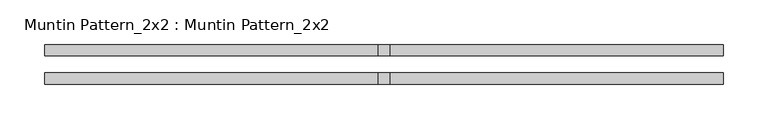
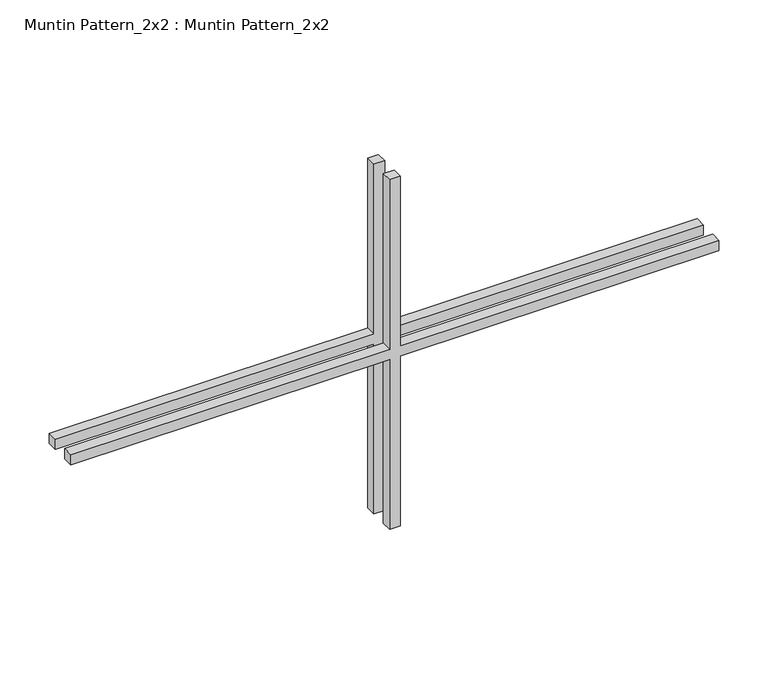
"""IFC4 building model written with IfcOpenShell, lengths in millimetres: proxy geometry, Muntin Pattern_2x2 : Muntin Pattern_2x2."""

from ifc_helpers import new_model, si_unit, frame, origin, place, context, project, spatial, polyline, outline, extrude, source, transform, mapped, element, save


def muntin_pattern_2x2_muntin_pattern_2x2_0e62f131(model_context):
    return source(origin(), model_context, "Body", "SweptSolid", [
        extrude(outline(polyline([(223.8375, -6.35), (223.8375, -381.0), (211.1375, -381.0), (211.1375, -6.35), (0.0, -6.35), (0.0, 6.35), (211.1375, 6.35), (211.1375, 381.0), (223.8375, 381.0), (223.8375, 6.35), (434.975, 6.35), (434.975, -6.35), (223.8375, -6.35)])), frame((0.0, 9.525, 0.0), z_axis=(0.0, 1.0, 0.0), x_axis=(0.0, 0.0, 1.0)), (0.0, 0.0, 1.0), 12.7),
        extrude(outline(polyline([(223.8375, -6.35), (223.8375, -381.0), (211.1375, -381.0), (211.1375, -6.35), (0.0, -6.35), (0.0, 6.35), (211.1375, 6.35), (211.1375, 381.0), (223.8375, 381.0), (223.8375, 6.35), (434.975, 6.35), (434.975, -6.35), (223.8375, -6.35)])), frame((0.0, -22.225, 0.0), z_axis=(0.0, 1.0, 0.0), x_axis=(0.0, 0.0, 1.0)), (0.0, 0.0, 1.0), 12.7),
    ])


if __name__ == "__main__":
    model = new_model("IFC4")
    model_context = context("Model", 3, world=origin())
    ifc_project = project(units=[si_unit("LENGTHUNIT", "METRE", prefix="MILLI")], contexts=[model_context])
    site = spatial("IfcSite", under=ifc_project)
    building = spatial("IfcBuilding", under=site)
    placement = place(None, origin())
    muntin_pattern_2x2_muntin_pattern_2x2_shape = muntin_pattern_2x2_muntin_pattern_2x2_0e62f131(model_context)
    element("IfcBuildingElementProxy", 1, Name="Muntin Pattern_2x2 : Muntin Pattern_2x2", ObjectType="Muntin Pattern_2x2 : Muntin Pattern_2x2", at=placement, inside=building, context=model_context, shape_type="MappedRepresentation", body=[
        mapped(muntin_pattern_2x2_muntin_pattern_2x2_shape, transform((0.0, 0.0, 0.0), x_axis=(1.0, 0.0, 0.0), y_axis=(0.0, 1.0, 0.0), z_axis=(0.0, 0.0, 1.0))),
    ])
    save(model, "model.ifc")

# Revit data of these elements
# Type "Muntin Pattern_2x2 : Muntin Pattern_2x2"
#   Width [instance default] = 4' - 0"
#   Thickness = 0' - 0 1/2"
#   Height [instance default] = 4' - 0"
#   Distance = 0' - 0 3/4"
#   Interior Material [instance default] = none
#   Exterior Material [instance default] = none
#   Default Elevation = 0
# Element 1 (IfcBuildingElementProxy, "Muntin Pattern_2x2 : Muntin Pattern_2x2")
#   Width = 2' - 6"
#   Height = 1' - 5 1/8"
#   Interior Material = Wood - Stained
#   Exterior Material = Clad - White
#   Materials on its faces: "Clad - White", "Wood - Stained"
# Materials
#   "Clad - White": class "Wood", colour RGB 242 242 238, transparency 0, Cost = 0
#   "Wood - Stained": class "Wood", colour RGB 224 178 126, transparency 0, Cost = 0
